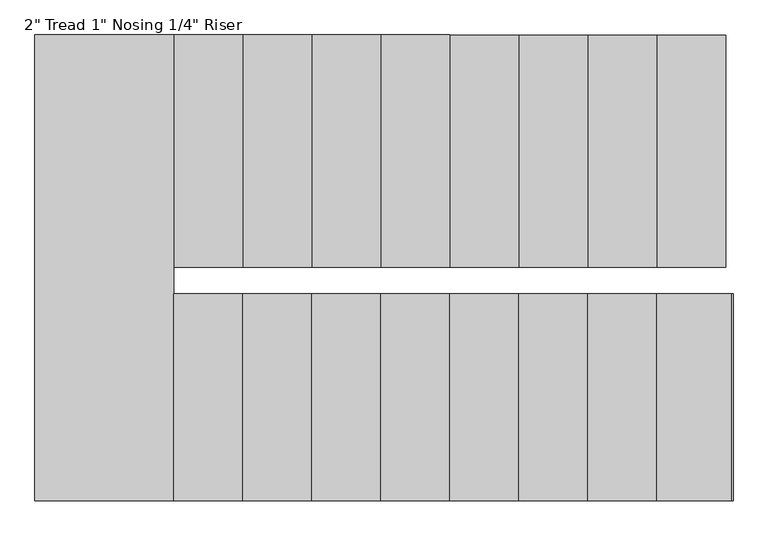
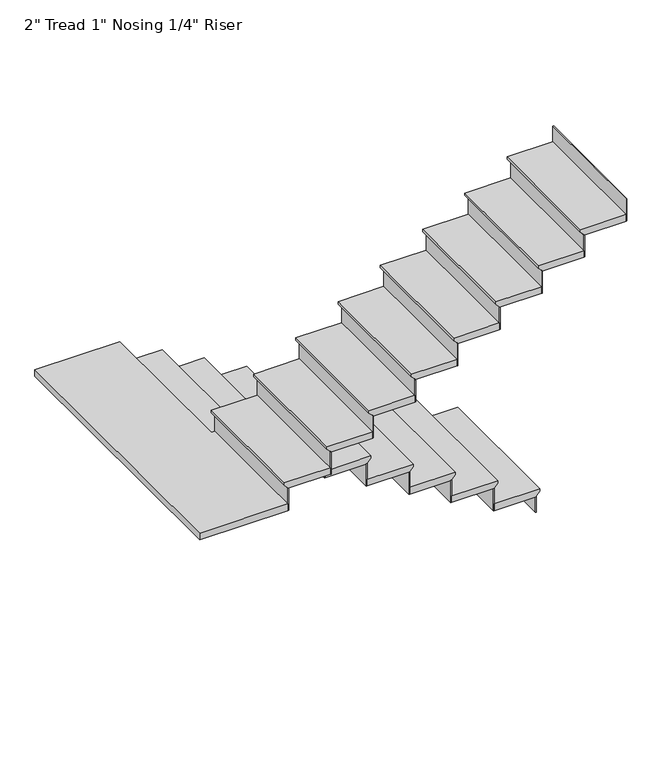
"""IFC4 building model written with IfcOpenShell, lengths in millimetres: stair flight geometry."""

from ifc_helpers import new_model, si_unit, origin, place, context, project, spatial, faceted_brep, source, transform, mapped, element, save


def stair_flight_597ccfed(model_context):
    return source(origin(), model_context, "Body", "Brep", [
        faceted_brep([(4295.1355783, 9969.5, 15390.2833333), (4295.1355783, 9969.5, 15409.3333333), (4295.1355783, 8944.6068332, 15409.3333333), (4295.1355783, 8944.6068332, 15390.2833333), (4269.7355783, 9969.5, 15364.8833333), (4269.7355783, 8944.6068332, 15364.8833333), (3964.9355783, 9969.5, 15409.3333333), (3964.9355783, 8944.6068332, 15409.3333333), (4269.7355783, 8944.6068332, 15358.5333333), (3964.9355783, 8944.6068332, 15358.5333333), (3964.9355783, 9969.5, 15358.5333333), (4269.7355783, 9969.5, 15358.5333333)], [[[0, 1, 2, 3]], [[4, 0, 3, 5]], [[2, 1, 6, 7]], [[8, 9, 10, 11]], [[2, 7, 9, 8, 5, 3]], [[8, 11, 4, 5]], [[6, 1, 0, 4, 11, 10]], [[7, 6, 10, 9]]]),
        faceted_brep([(4269.7355783, 9969.5, 15358.5333333), (4269.7355783, 9969.5, 15240.0), (4263.3855783, 9969.5, 15240.0), (4263.3855783, 9969.5, 15358.5333333), (4269.7355783, 8944.6068332, 15358.5333333), (4263.3855783, 8944.6068332, 15358.5333333), (4263.3855783, 8944.6068332, 15240.0), (4269.7355783, 8944.6068332, 15240.0)], [[[0, 1, 2, 3]], [[4, 5, 6, 7]], [[1, 0, 4, 7]], [[2, 1, 7, 6]], [[3, 2, 6, 5]], [[0, 3, 5, 4]]]),
        faceted_brep([(3964.9355783, 9969.5, 15527.8666667), (3964.9355783, 9969.5, 15358.5333333), (3958.5855783, 9969.5, 15358.5333333), (3958.5855783, 9969.5, 15527.8666667), (3964.9355783, 8944.6068332, 15527.8666667), (3958.5855783, 8944.6068332, 15527.8666667), (3958.5855783, 8944.6068332, 15358.5333333), (3964.9355783, 8944.6068332, 15358.5333333)], [[[0, 1, 2, 3]], [[4, 5, 6, 7]], [[1, 0, 4, 7]], [[2, 1, 7, 6]], [[3, 2, 6, 5]], [[0, 3, 5, 4]]]),
        faceted_brep([(3990.3355783, 8944.6068332, 15578.6666667), (3990.3355783, 9969.5, 15578.6666667), (3660.1355783, 9969.5, 15578.6666667), (3660.1355783, 8944.6068332, 15578.6666667), (3964.9355783, 8944.6068332, 15527.8666667), (3660.1355783, 8944.6068332, 15527.8666667), (3660.1355783, 9969.5, 15527.8666667), (3964.9355783, 9969.5, 15527.8666667), (3964.9355783, 8944.6068332, 15534.2166667), (3990.3355783, 8944.6068332, 15559.6166667), (3964.9355783, 9969.5, 15534.2166667), (3990.3355783, 9969.5, 15559.6166667)], [[[0, 1, 2, 3]], [[4, 5, 6, 7]], [[0, 3, 5, 4, 8, 9]], [[4, 7, 10, 8]], [[2, 1, 11, 10, 7, 6]], [[3, 2, 6, 5]], [[11, 1, 0, 9]], [[10, 11, 9, 8]]]),
        faceted_brep([(3660.1355783, 9969.5, 15697.2), (3660.1355783, 9969.5, 15527.8666667), (3653.7855783, 9969.5, 15527.8666667), (3653.7855783, 9969.5, 15697.2), (3660.1355783, 8944.6068332, 15697.2), (3653.7855783, 8944.6068332, 15697.2), (3653.7855783, 8944.6068332, 15527.8666667), (3660.1355783, 8944.6068332, 15527.8666667)], [[[0, 1, 2, 3]], [[4, 5, 6, 7]], [[1, 0, 4, 7]], [[2, 1, 7, 6]], [[3, 2, 6, 5]], [[0, 3, 5, 4]]]),
        faceted_brep([(3685.5355783, 8944.6068332, 15748.0), (3685.5355783, 9969.5, 15748.0), (3355.3355783, 9969.5, 15748.0), (3355.3355783, 8944.6068332, 15748.0), (3660.1355783, 8944.6068332, 15697.2), (3355.3355783, 8944.6068332, 15697.2), (3355.3355783, 9969.5, 15697.2), (3660.1355783, 9969.5, 15697.2), (3660.1355783, 8944.6068332, 15703.55), (3685.5355783, 8944.6068332, 15728.95), (3660.1355783, 9969.5, 15703.55), (3685.5355783, 9969.5, 15728.95)], [[[0, 1, 2, 3]], [[4, 5, 6, 7]], [[0, 3, 5, 4, 8, 9]], [[4, 7, 10, 8]], [[2, 1, 11, 10, 7, 6]], [[3, 2, 6, 5]], [[11, 1, 0, 9]], [[10, 11, 9, 8]]]),
        faceted_brep([(3355.3355783, 9969.5, 15866.5333333), (3355.3355783, 9969.5, 15697.2), (3348.9855783, 9969.5, 15697.2), (3348.9855783, 9969.5, 15866.5333333), (3355.3355783, 8944.6068332, 15866.5333333), (3348.9855783, 8944.6068332, 15866.5333333), (3348.9855783, 8944.6068332, 15697.2), (3355.3355783, 8944.6068332, 15697.2)], [[[0, 1, 2, 3]], [[4, 5, 6, 7]], [[1, 0, 4, 7]], [[2, 1, 7, 6]], [[3, 2, 6, 5]], [[0, 3, 5, 4]]]),
        faceted_brep([(3380.7355783, 8944.6068332, 15917.3333333), (3380.7355783, 9969.5, 15917.3333333), (3050.5355783, 9969.5, 15917.3333333), (3050.5355783, 8944.6068332, 15917.3333333), (3355.3355783, 8944.6068332, 15866.5333333), (3050.5355783, 8944.6068332, 15866.5333333), (3050.5355783, 9969.5, 15866.5333333), (3355.3355783, 9969.5, 15866.5333333), (3355.3355783, 8944.6068332, 15872.8833333), (3380.7355783, 8944.6068332, 15898.2833333), (3355.3355783, 9969.5, 15872.8833333), (3380.7355783, 9969.5, 15898.2833333)], [[[0, 1, 2, 3]], [[4, 5, 6, 7]], [[0, 3, 5, 4, 8, 9]], [[4, 7, 10, 8]], [[2, 1, 11, 10, 7, 6]], [[3, 2, 6, 5]], [[11, 1, 0, 9]], [[10, 11, 9, 8]]]),
        faceted_brep([(3050.5355783, 9969.5, 16035.8666667), (3050.5355783, 9969.5, 15866.5333333), (3044.1855783, 9969.5, 15866.5333333), (3044.1855783, 9969.5, 16035.8666667), (3050.5355783, 8944.6068332, 16035.8666667), (3044.1855783, 8944.6068332, 16035.8666667), (3044.1855783, 8944.6068332, 15866.5333333), (3050.5355783, 8944.6068332, 15866.5333333)], [[[0, 1, 2, 3]], [[4, 5, 6, 7]], [[1, 0, 4, 7]], [[2, 1, 7, 6]], [[3, 2, 6, 5]], [[0, 3, 5, 4]]]),
        faceted_brep([(3075.9355783, 8944.6068332, 16086.6666667), (3075.9355783, 9969.5, 16086.6666667), (2745.7355783, 9969.5, 16086.6666667), (2745.7355783, 8944.6068332, 16086.6666667), (3050.5355783, 8944.6068332, 16035.8666667), (2745.7355783, 8944.6068332, 16035.8666667), (2745.7355783, 9969.5, 16035.8666667), (3050.5355783, 9969.5, 16035.8666667), (3050.5355783, 8944.6068332, 16042.2166667), (3075.9355783, 8944.6068332, 16067.6166667), (3050.5355783, 9969.5, 16042.2166667), (3075.9355783, 9969.5, 16067.6166667)], [[[0, 1, 2, 3]], [[4, 5, 6, 7]], [[0, 3, 5, 4, 8, 9]], [[4, 7, 10, 8]], [[2, 1, 11, 10, 7, 6]], [[3, 2, 6, 5]], [[11, 1, 0, 9]], [[10, 11, 9, 8]]]),
        faceted_brep([(2745.7355783, 9969.5, 16205.2), (2745.7355783, 9969.5, 16035.8666667), (2739.3855783, 9969.5, 16035.8666667), (2739.3855783, 9969.5, 16205.2), (2745.7355783, 8944.6068332, 16205.2), (2739.3855783, 8944.6068332, 16205.2), (2739.3855783, 8944.6068332, 16035.8666667), (2745.7355783, 8944.6068332, 16035.8666667)], [[[0, 1, 2, 3]], [[4, 5, 6, 7]], [[1, 0, 4, 7]], [[2, 1, 7, 6]], [[3, 2, 6, 5]], [[0, 3, 5, 4]]]),
        faceted_brep([(2771.1355783, 8944.6068332, 16256.0), (2771.1355783, 9969.5, 16256.0), (2440.9355783, 9969.5, 16256.0), (2440.9355783, 8944.6068332, 16256.0), (2745.7355783, 8944.6068332, 16205.2), (2440.9355783, 8944.6068332, 16205.2), (2440.9355783, 9969.5, 16205.2), (2745.7355783, 9969.5, 16205.2), (2745.7355783, 8944.6068332, 16211.55), (2771.1355783, 8944.6068332, 16236.95), (2745.7355783, 9969.5, 16211.55), (2771.1355783, 9969.5, 16236.95)], [[[0, 1, 2, 3]], [[4, 5, 6, 7]], [[0, 3, 5, 4, 8, 9]], [[4, 7, 10, 8]], [[2, 1, 11, 10, 7, 6]], [[3, 2, 6, 5]], [[11, 1, 0, 9]], [[10, 11, 9, 8]]]),
        faceted_brep([(2440.9355783, 9969.5, 16374.5333333), (2440.9355783, 9969.5, 16205.2), (2434.5855783, 9969.5, 16205.2), (2434.5855783, 9969.5, 16374.5333333), (2440.9355783, 8944.6068332, 16374.5333333), (2434.5855783, 8944.6068332, 16374.5333333), (2434.5855783, 8944.6068332, 16205.2), (2440.9355783, 8944.6068332, 16205.2)], [[[0, 1, 2, 3]], [[4, 5, 6, 7]], [[1, 0, 4, 7]], [[2, 1, 7, 6]], [[3, 2, 6, 5]], [[0, 3, 5, 4]]]),
        faceted_brep([(2466.3355783, 8944.6068332, 16425.3333333), (2466.3355783, 9969.5, 16425.3333333), (2136.1355783, 9969.5, 16425.3333333), (2136.1355783, 8944.6068332, 16425.3333333), (2440.9355783, 8944.6068332, 16374.5333333), (2136.1355783, 8944.6068332, 16374.5333333), (2136.1355783, 9969.5, 16374.5333333), (2440.9355783, 9969.5, 16374.5333333), (2440.9355783, 8944.6068332, 16380.8833333), (2466.3355783, 8944.6068332, 16406.2833333), (2440.9355783, 9969.5, 16380.8833333), (2466.3355783, 9969.5, 16406.2833333)], [[[0, 1, 2, 3]], [[4, 5, 6, 7]], [[0, 3, 5, 4, 8, 9]], [[4, 7, 10, 8]], [[2, 1, 11, 10, 7, 6]], [[3, 2, 6, 5]], [[11, 1, 0, 9]], [[10, 11, 9, 8]]]),
        faceted_brep([(2136.1355783, 9969.5, 16543.8666667), (2136.1355783, 9969.5, 16374.5333333), (2129.7855783, 9969.5, 16374.5333333), (2129.7855783, 9969.5, 16543.8666667), (2136.1355783, 8944.6068332, 16543.8666667), (2129.7855783, 8944.6068332, 16543.8666667), (2129.7855783, 8944.6068332, 16374.5333333), (2136.1355783, 8944.6068332, 16374.5333333)], [[[0, 1, 2, 3]], [[4, 5, 6, 7]], [[1, 0, 4, 7]], [[2, 1, 7, 6]], [[3, 2, 6, 5]], [[0, 3, 5, 4]]]),
        faceted_brep([(2161.5355783, 8944.6068332, 16594.6666667), (2161.5355783, 9969.5, 16594.6666667), (1831.3355783, 9969.5, 16594.6666667), (1831.3355783, 8944.6068332, 16594.6666667), (2136.1355783, 8944.6068332, 16543.8666667), (1831.3355783, 8944.6068332, 16543.8666667), (1831.3355783, 9969.5, 16543.8666667), (2136.1355783, 9969.5, 16543.8666667), (2136.1355783, 8944.6068332, 16550.2166667), (2161.5355783, 8944.6068332, 16575.6166667), (2136.1355783, 9969.5, 16550.2166667), (2161.5355783, 9969.5, 16575.6166667)], [[[0, 1, 2, 3]], [[4, 5, 6, 7]], [[0, 3, 5, 4, 8, 9]], [[4, 7, 10, 8]], [[2, 1, 11, 10, 7, 6]], [[3, 2, 6, 5]], [[11, 1, 0, 9]], [[10, 11, 9, 8]]]),
        faceted_brep([(1831.3355783, 9969.5, 16713.2), (1831.3355783, 9969.5, 16543.8666667), (1824.9855783, 9969.5, 16543.8666667), (1824.9855783, 9969.5, 16713.2), (1831.3355783, 8944.6068332, 16713.2), (1824.9855783, 8944.6068332, 16713.2), (1824.9855783, 8944.6068332, 16543.8666667), (1831.3355783, 8944.6068332, 16543.8666667)], [[[0, 1, 2, 3]], [[4, 5, 6, 7]], [[1, 0, 4, 7]], [[2, 1, 7, 6]], [[3, 2, 6, 5]], [[0, 3, 5, 4]]]),
        faceted_brep([(1882.1355783, 8826.5, 16764.0), (1856.7355783, 8826.5, 16764.0), (1856.7355783, 9969.5, 16764.0), (1244.6, 9969.5, 16764.0), (1244.6, 7912.1, 16764.0), (1882.1355783, 7912.1, 16764.0), (1856.7355783, 8826.5, 16713.2), (1882.1355783, 8826.5, 16713.2), (1882.1355783, 7912.1, 16713.2), (1244.6, 7912.1, 16713.2), (1244.6, 9969.5, 16713.2), (1831.3355783, 9969.5, 16713.2), (1831.3355783, 8944.6068332, 16713.2), (1856.7355783, 8944.6068332, 16713.2), (1856.7355783, 8944.6068332, 16744.95), (1856.7355783, 9969.5, 16744.95), (1831.3355783, 8944.6068332, 16719.55), (1831.3355783, 9969.5, 16719.55)], [[[0, 1, 2, 3, 4, 5]], [[6, 7, 8, 9, 10, 11, 12, 13]], [[1, 0, 7, 6]], [[2, 1, 6, 13, 14, 15]], [[13, 12, 16, 14]], [[12, 11, 17, 16]], [[3, 2, 15, 17, 11, 10]], [[4, 3, 10, 9]], [[5, 4, 9, 8]], [[0, 5, 8, 7]], [[17, 15, 14, 16]]]),
        faceted_brep([(1882.1355783, 7912.1, 16882.5333333), (1882.1355783, 7912.1, 16713.2), (1888.4855783, 7912.1, 16713.2), (1888.4855783, 7912.1, 16882.5333333), (1882.1355783, 8826.5, 16882.5333333), (1888.4855783, 8826.5, 16882.5333333), (1888.4855783, 8826.5, 16713.2), (1882.1355783, 8826.5, 16713.2)], [[[0, 1, 2, 3]], [[4, 5, 6, 7]], [[1, 0, 4, 7]], [[2, 1, 7, 6]], [[3, 2, 6, 5]], [[0, 3, 5, 4]]]),
        faceted_brep([(1856.7355783, 8826.5, 16933.3333333), (1856.7355783, 7912.1, 16933.3333333), (2186.9355783, 7912.1, 16933.3333333), (2186.9355783, 8826.5, 16933.3333333), (1882.1355783, 8826.5, 16882.5333333), (2186.9355783, 8826.5, 16882.5333333), (2186.9355783, 7912.1, 16882.5333333), (1882.1355783, 7912.1, 16882.5333333), (1882.1355783, 8826.5, 16888.8833333), (1856.7355783, 8826.5, 16914.2833333), (1882.1355783, 7912.1, 16888.8833333), (1856.7355783, 7912.1, 16914.2833333)], [[[0, 1, 2, 3]], [[4, 5, 6, 7]], [[0, 3, 5, 4, 8, 9]], [[4, 7, 10, 8]], [[2, 1, 11, 10, 7, 6]], [[3, 2, 6, 5]], [[11, 1, 0, 9]], [[10, 11, 9, 8]]]),
        faceted_brep([(2186.9355783, 7912.1, 17051.8666667), (2186.9355783, 7912.1, 16882.5333333), (2193.2855783, 7912.1, 16882.5333333), (2193.2855783, 7912.1, 17051.8666667), (2186.9355783, 8826.5, 17051.8666667), (2193.2855783, 8826.5, 17051.8666667), (2193.2855783, 8826.5, 16882.5333333), (2186.9355783, 8826.5, 16882.5333333)], [[[0, 1, 2, 3]], [[4, 5, 6, 7]], [[1, 0, 4, 7]], [[2, 1, 7, 6]], [[3, 2, 6, 5]], [[0, 3, 5, 4]]]),
        faceted_brep([(2161.5355783, 8826.5, 17102.6666667), (2161.5355783, 7912.1, 17102.6666667), (2491.7355783, 7912.1, 17102.6666667), (2491.7355783, 8826.5, 17102.6666667), (2186.9355783, 8826.5, 17051.8666667), (2491.7355783, 8826.5, 17051.8666667), (2491.7355783, 7912.1, 17051.8666667), (2186.9355783, 7912.1, 17051.8666667), (2186.9355783, 8826.5, 17058.2166667), (2161.5355783, 8826.5, 17083.6166667), (2186.9355783, 7912.1, 17058.2166667), (2161.5355783, 7912.1, 17083.6166667)], [[[0, 1, 2, 3]], [[4, 5, 6, 7]], [[0, 3, 5, 4, 8, 9]], [[4, 7, 10, 8]], [[2, 1, 11, 10, 7, 6]], [[3, 2, 6, 5]], [[11, 1, 0, 9]], [[10, 11, 9, 8]]]),
        faceted_brep([(2491.7355783, 7912.1, 17221.2), (2491.7355783, 7912.1, 17051.8666667), (2498.0855783, 7912.1, 17051.8666667), (2498.0855783, 7912.1, 17221.2), (2491.7355783, 8826.5, 17221.2), (2498.0855783, 8826.5, 17221.2), (2498.0855783, 8826.5, 17051.8666667), (2491.7355783, 8826.5, 17051.8666667)], [[[0, 1, 2, 3]], [[4, 5, 6, 7]], [[1, 0, 4, 7]], [[2, 1, 7, 6]], [[3, 2, 6, 5]], [[0, 3, 5, 4]]]),
        faceted_brep([(2466.3355783, 8826.5, 17272.0), (2466.3355783, 7912.1, 17272.0), (2796.5355783, 7912.1, 17272.0), (2796.5355783, 8826.5, 17272.0), (2491.7355783, 8826.5, 17221.2), (2796.5355783, 8826.5, 17221.2), (2796.5355783, 7912.1, 17221.2), (2491.7355783, 7912.1, 17221.2), (2491.7355783, 8826.5, 17227.55), (2466.3355783, 8826.5, 17252.95), (2491.7355783, 7912.1, 17227.55), (2466.3355783, 7912.1, 17252.95)], [[[0, 1, 2, 3]], [[4, 5, 6, 7]], [[0, 3, 5, 4, 8, 9]], [[4, 7, 10, 8]], [[2, 1, 11, 10, 7, 6]], [[3, 2, 6, 5]], [[11, 1, 0, 9]], [[10, 11, 9, 8]]]),
        faceted_brep([(2796.5355783, 7912.1, 17390.5333333), (2796.5355783, 7912.1, 17221.2), (2802.8855783, 7912.1, 17221.2), (2802.8855783, 7912.1, 17390.5333333), (2796.5355783, 8826.5, 17390.5333333), (2802.8855783, 8826.5, 17390.5333333), (2802.8855783, 8826.5, 17221.2), (2796.5355783, 8826.5, 17221.2)], [[[0, 1, 2, 3]], [[4, 5, 6, 7]], [[1, 0, 4, 7]], [[2, 1, 7, 6]], [[3, 2, 6, 5]], [[0, 3, 5, 4]]]),
        faceted_brep([(2771.1355783, 8826.5, 17441.3333333), (2771.1355783, 7912.1, 17441.3333333), (3101.3355783, 7912.1, 17441.3333333), (3101.3355783, 8826.5, 17441.3333333), (2796.5355783, 8826.5, 17390.5333333), (3101.3355783, 8826.5, 17390.5333333), (3101.3355783, 7912.1, 17390.5333333), (2796.5355783, 7912.1, 17390.5333333), (2796.5355783, 8826.5, 17396.8833333), (2771.1355783, 8826.5, 17422.2833333), (2796.5355783, 7912.1, 17396.8833333), (2771.1355783, 7912.1, 17422.2833333)], [[[0, 1, 2, 3]], [[4, 5, 6, 7]], [[0, 3, 5, 4, 8, 9]], [[4, 7, 10, 8]], [[2, 1, 11, 10, 7, 6]], [[3, 2, 6, 5]], [[11, 1, 0, 9]], [[10, 11, 9, 8]]]),
        faceted_brep([(3101.3355783, 7912.1, 17559.8666667), (3101.3355783, 7912.1, 17390.5333333), (3107.6855783, 7912.1, 17390.5333333), (3107.6855783, 7912.1, 17559.8666667), (3101.3355783, 8826.5, 17559.8666667), (3107.6855783, 8826.5, 17559.8666667), (3107.6855783, 8826.5, 17390.5333333), (3101.3355783, 8826.5, 17390.5333333)], [[[0, 1, 2, 3]], [[4, 5, 6, 7]], [[1, 0, 4, 7]], [[2, 1, 7, 6]], [[3, 2, 6, 5]], [[0, 3, 5, 4]]]),
        faceted_brep([(3075.9355783, 8826.5, 17610.6666667), (3075.9355783, 7912.1, 17610.6666667), (3406.1355783, 7912.1, 17610.6666667), (3406.1355783, 8826.5, 17610.6666667), (3101.3355783, 8826.5, 17559.8666667), (3406.1355783, 8826.5, 17559.8666667), (3406.1355783, 7912.1, 17559.8666667), (3101.3355783, 7912.1, 17559.8666667), (3101.3355783, 8826.5, 17566.2166667), (3075.9355783, 8826.5, 17591.6166667), (3101.3355783, 7912.1, 17566.2166667), (3075.9355783, 7912.1, 17591.6166667)], [[[0, 1, 2, 3]], [[4, 5, 6, 7]], [[0, 3, 5, 4, 8, 9]], [[4, 7, 10, 8]], [[2, 1, 11, 10, 7, 6]], [[3, 2, 6, 5]], [[11, 1, 0, 9]], [[10, 11, 9, 8]]]),
        faceted_brep([(3406.1355783, 7912.1, 17729.2), (3406.1355783, 7912.1, 17559.8666667), (3412.4855783, 7912.1, 17559.8666667), (3412.4855783, 7912.1, 17729.2), (3406.1355783, 8826.5, 17729.2), (3412.4855783, 8826.5, 17729.2), (3412.4855783, 8826.5, 17559.8666667), (3406.1355783, 8826.5, 17559.8666667)], [[[0, 1, 2, 3]], [[4, 5, 6, 7]], [[1, 0, 4, 7]], [[2, 1, 7, 6]], [[3, 2, 6, 5]], [[0, 3, 5, 4]]]),
        faceted_brep([(3380.7355783, 8826.5, 17780.0), (3380.7355783, 7912.1, 17780.0), (3710.9355783, 7912.1, 17780.0), (3710.9355783, 8826.5, 17780.0), (3406.1355783, 8826.5, 17729.2), (3710.9355783, 8826.5, 17729.2), (3710.9355783, 7912.1, 17729.2), (3406.1355783, 7912.1, 17729.2), (3406.1355783, 8826.5, 17735.55), (3380.7355783, 8826.5, 17760.95), (3406.1355783, 7912.1, 17735.55), (3380.7355783, 7912.1, 17760.95)], [[[0, 1, 2, 3]], [[4, 5, 6, 7]], [[0, 3, 5, 4, 8, 9]], [[4, 7, 10, 8]], [[2, 1, 11, 10, 7, 6]], [[3, 2, 6, 5]], [[11, 1, 0, 9]], [[10, 11, 9, 8]]]),
        faceted_brep([(3710.9355783, 7912.1, 17898.5333333), (3710.9355783, 7912.1, 17729.2), (3717.2855783, 7912.1, 17729.2), (3717.2855783, 7912.1, 17898.5333333), (3710.9355783, 8826.5, 17898.5333333), (3717.2855783, 8826.5, 17898.5333333), (3717.2855783, 8826.5, 17729.2), (3710.9355783, 8826.5, 17729.2)], [[[0, 1, 2, 3]], [[4, 5, 6, 7]], [[1, 0, 4, 7]], [[2, 1, 7, 6]], [[3, 2, 6, 5]], [[0, 3, 5, 4]]]),
        faceted_brep([(3685.5355783, 8826.5, 17949.3333333), (3685.5355783, 7912.1, 17949.3333333), (4015.7355783, 7912.1, 17949.3333333), (4015.7355783, 8826.5, 17949.3333333), (3710.9355783, 8826.5, 17898.5333333), (4015.7355783, 8826.5, 17898.5333333), (4015.7355783, 7912.1, 17898.5333333), (3710.9355783, 7912.1, 17898.5333333), (3710.9355783, 8826.5, 17904.8833333), (3685.5355783, 8826.5, 17930.2833333), (3710.9355783, 7912.1, 17904.8833333), (3685.5355783, 7912.1, 17930.2833333)], [[[0, 1, 2, 3]], [[4, 5, 6, 7]], [[0, 3, 5, 4, 8, 9]], [[4, 7, 10, 8]], [[2, 1, 11, 10, 7, 6]], [[3, 2, 6, 5]], [[11, 1, 0, 9]], [[10, 11, 9, 8]]]),
        faceted_brep([(4015.7355783, 7912.1, 18067.8666667), (4015.7355783, 7912.1, 17898.5333333), (4022.0855783, 7912.1, 17898.5333333), (4022.0855783, 7912.1, 18067.8666667), (4015.7355783, 8826.5, 18067.8666667), (4022.0855783, 8826.5, 18067.8666667), (4022.0855783, 8826.5, 17898.5333333), (4015.7355783, 8826.5, 17898.5333333)], [[[0, 1, 2, 3]], [[4, 5, 6, 7]], [[1, 0, 4, 7]], [[2, 1, 7, 6]], [[3, 2, 6, 5]], [[0, 3, 5, 4]]]),
        faceted_brep([(4320.5355783, 7912.1, 18237.2), (4320.5355783, 7912.1, 18067.8666667), (4326.8855783, 7912.1, 18067.8666667), (4326.8855783, 7912.1, 18237.2), (4320.5355783, 8826.5, 18237.2), (4326.8855783, 8826.5, 18237.2), (4326.8855783, 8826.5, 18067.8666667), (4320.5355783, 8826.5, 18067.8666667)], [[[0, 1, 2, 3]], [[4, 5, 6, 7]], [[1, 0, 4, 7]], [[2, 1, 7, 6]], [[3, 2, 6, 5]], [[0, 3, 5, 4]]]),
        faceted_brep([(3990.3355783, 8826.5, 18118.6666667), (3990.3355783, 7912.1, 18118.6666667), (4320.5355783, 7912.1, 18118.6666667), (4320.5355783, 8826.5, 18118.6666667), (4015.7355783, 8826.5, 18067.8666667), (4320.5355783, 8826.5, 18067.8666667), (4320.5355783, 7912.1, 18067.8666667), (4015.7355783, 7912.1, 18067.8666667), (4015.7355783, 8826.5, 18074.2166667), (3990.3355783, 8826.5, 18099.6166667), (4015.7355783, 7912.1, 18074.2166667), (3990.3355783, 7912.1, 18099.6166667)], [[[0, 1, 2, 3]], [[4, 5, 6, 7]], [[0, 3, 5, 4, 8, 9]], [[4, 7, 10, 8]], [[2, 1, 11, 10, 7, 6]], [[3, 2, 6, 5]], [[11, 1, 0, 9]], [[10, 11, 9, 8]]]),
    ])


if __name__ == "__main__":
    model = new_model("IFC4")
    model_context = context("Model", 3, world=origin())
    ifc_project = project(units=[si_unit("LENGTHUNIT", "METRE", prefix="MILLI")], contexts=[model_context])
    site = spatial("IfcSite", under=ifc_project)
    building = spatial("IfcBuilding", under=site)
    placement = place(None, origin())
    stair_flight_shape = stair_flight_597ccfed(model_context)
    element("IfcStairFlight", 1, ObjectType="2\" Tread 1\" Nosing 1/4\" Riser", at=placement, inside=building, context=model_context, shape_type="MappedRepresentation", body=[
        mapped(stair_flight_shape, transform((0.0, 0.0, 0.0), x_axis=(1.0, 0.0, 0.0), y_axis=(0.0, 1.0, 0.0), z_axis=(0.0, 0.0, 1.0))),
    ])
    save(model, "model.ifc")
